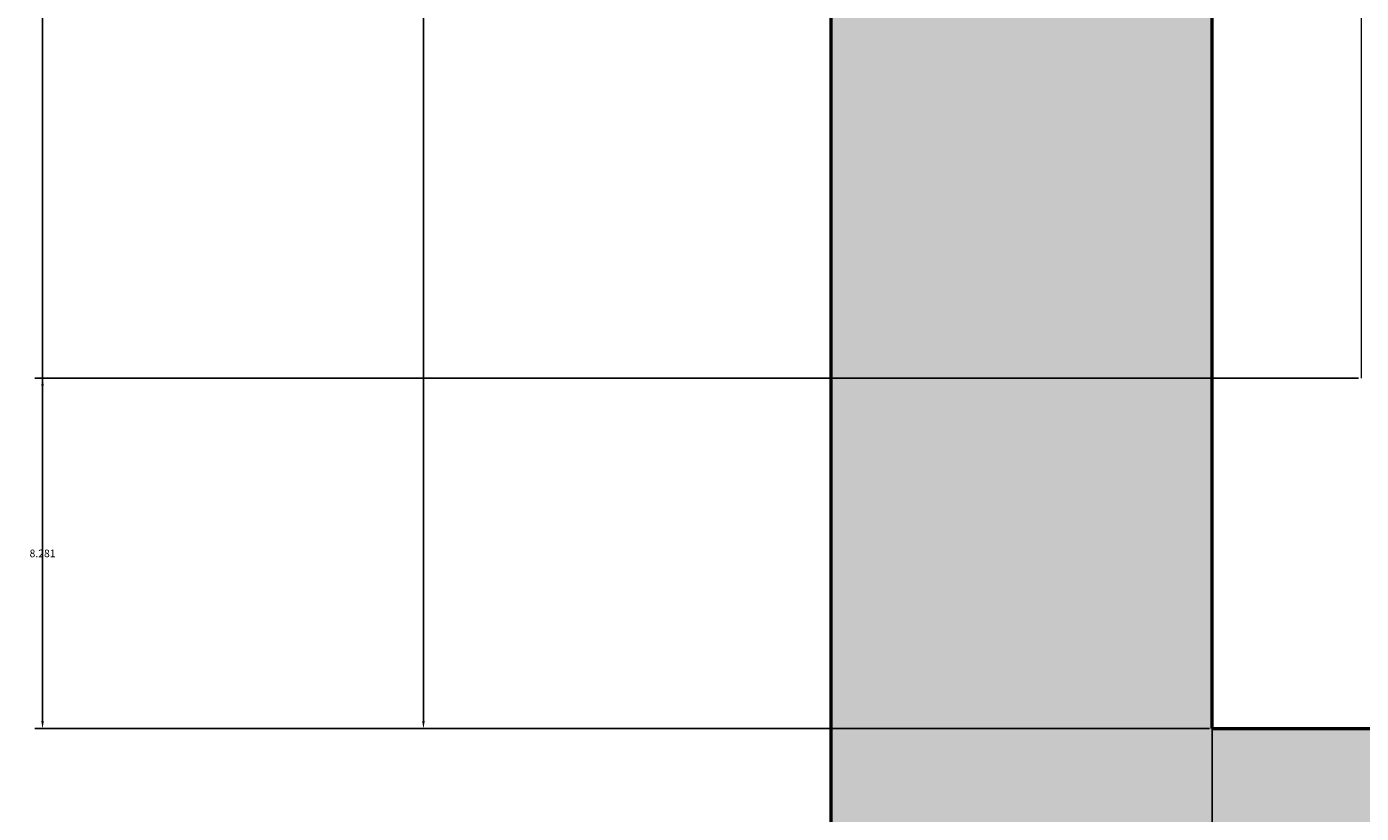
# Model space of a CAD drawing. Units: inches. Extents: x 2231 to 2461, y 2045 to 2455.
# Tile 36 of 95: x 2231 to 2262, y 2185 to 2203. Entities that reach past the tile are written whole.
import ezdxf

# ---------------------------------------------------------------- set-up
doc = ezdxf.new("R2010")
doc.units = ezdxf.units.IN
for name, color, linetype, lineweight in [('A-ANNO-DIMS', 2, 'Continuous', 18), ('A-FURN', 9, 'Continuous', 18), ('A-WALL', 7, 'Continuous', 50)]:
    doc.layers.add(name, color=color, linetype=linetype, lineweight=lineweight)
doc.layers.add('A-WALL-PATT', color=18, linetype='Continuous', lineweight=13, true_color=0x000000)
doc.styles.get("Standard").update_dxf_attribs({"font": 'arial.ttf'})
doc.dimstyles.get("Standard").update_dxf_attribs({"dimtxt": 0.18, "dimasz": 0.18, "dimexe": 0.18, "dimexo": 0.0625, "dimgap": 0.09, "dimtad": 0, "dimtih": 1, "dimtoh": 1, "dimdec": 4, "dimzin": 0, "dimdsep": 46, "dimtxsty": 'Standard', "dimcen": 0.09, "dimadec": 0, "dimazin": 0, "dimtfac": 1, "dimtdec": 4, "dimtofl": 0, "dimtmove": 0, "dimatfit": 3, "dimfxl": 1, "dimtolj": 1, "dimtzin": 0, "dimarcsym": 0})

# ---------------------------------------------------------------- blocks, each defined once
blk = doc.blocks.new('*D39')
at = {"layer": 'A-ANNO-DIMS', "color": 0, "lineweight": -2, "transparency": 16777216}
for p, q in [((2258.731, 2221.999), (2230.981, 2221.999)), ((2231.161, 2221.819), (2231.161, 2204.598)), ((2231.161, 2187.013), (2231.161, 2204.234)), ((2258.731, 2186.833), (2230.981, 2186.833))]:
    blk.add_line(p, q, dxfattribs=at)
at = {"layer": 'A-ANNO-DIMS', "color": 0, "transparency": 16777216}
for points in [[(2231.131, 2221.819), (2231.191, 2221.819), (2231.161, 2221.999)], [(2231.131, 2187.013), (2231.191, 2187.013), (2231.161, 2186.833)]]:
    blk.add_solid(points, dxfattribs=at)
at = {"layer": 'Defpoints', "color": 0, "transparency": 16777216}
for p in [(2231.161, 2221.999), (2258.794, 2221.999), (2258.794, 2186.833)]:
    blk.add_point(p, dxfattribs=at)
at = {"layer": 'A-ANNO-DIMS', "color": 0, "transparency": 16777216, "insert": (2231.161, 2204.416), "char_height": 0.18, "attachment_point": 5}
blk.add_mtext('\\A1;35.166', dxfattribs=at)
blk = doc.blocks.new('*D40')
at = {"layer": 'A-ANNO-DIMS', "color": 0, "lineweight": -2, "transparency": 16777216}
for p, q in [((2258.731, 2302.833), (2239.981, 2302.833)), ((2240.161, 2302.653), (2240.161, 2245.015)), ((2240.161, 2187.013), (2240.161, 2244.651)), ((2258.731, 2186.833), (2239.981, 2186.833))]:
    blk.add_line(p, q, dxfattribs=at)
at = {"layer": 'A-ANNO-DIMS', "color": 0, "transparency": 16777216}
for points in [[(2240.131, 2302.653), (2240.191, 2302.653), (2240.161, 2302.833)], [(2240.131, 2187.013), (2240.191, 2187.013), (2240.161, 2186.833)]]:
    blk.add_solid(points, dxfattribs=at)
at = {"layer": 'Defpoints', "color": 0, "transparency": 16777216}
for p in [(2240.161, 2302.833), (2258.794, 2302.833), (2258.794, 2186.833)]:
    blk.add_point(p, dxfattribs=at)
at = {"layer": 'A-ANNO-DIMS', "color": 0, "transparency": 16777216, "insert": (2240.161, 2244.833), "char_height": 0.18, "attachment_point": 5}
blk.add_mtext('\\A1;116', dxfattribs=at)
blk = doc.blocks.new('*D47')
at = {"layer": 'A-ANNO-DIMS', "color": 0, "lineweight": -2, "transparency": 16777216}
for p, q in [((2258.794, 2182.895), (2258.794, 2454.645)), ((2258.974, 2454.465), (2276.575, 2454.465)), ((2294.614, 2454.465), (2277.012, 2454.465)), ((2294.794, 2182.895), (2294.794, 2454.645))]:
    blk.add_line(p, q, dxfattribs=at)
at = {"layer": 'A-ANNO-DIMS', "color": 0, "transparency": 16777216}
for points in [[(2258.974, 2454.495), (2258.974, 2454.435), (2258.794, 2454.465)], [(2294.614, 2454.495), (2294.614, 2454.435), (2294.794, 2454.465)]]:
    blk.add_solid(points, dxfattribs=at)
at = {"layer": 'Defpoints', "color": 0, "transparency": 16777216}
for p in [(2294.794, 2454.465), (2258.794, 2182.833), (2294.794, 2182.833)]:
    blk.add_point(p, dxfattribs=at)
at = {"layer": 'A-ANNO-DIMS', "color": 0, "transparency": 16777216, "insert": (2276.794, 2454.465), "char_height": 0.18, "attachment_point": 5}
blk.add_mtext('\\A1;36', dxfattribs=at)
blk = doc.blocks.new('*D51')
at = {"layer": 'A-ANNO-DIMS', "color": 0, "lineweight": -2, "transparency": 16777216}
for p, q in [((2258.794, 2306.77), (2258.794, 2044.803)), ((2330.794, 2306.77), (2330.794, 2044.803)), ((2258.974, 2044.983), (2294.576, 2044.983)), ((2330.614, 2044.983), (2295.011, 2044.983))]:
    blk.add_line(p, q, dxfattribs=at)
at = {"layer": 'A-ANNO-DIMS', "color": 0, "transparency": 16777216}
for points in [[(2258.974, 2045.013), (2258.974, 2044.953), (2258.794, 2044.983)], [(2330.614, 2045.013), (2330.614, 2044.953), (2330.794, 2044.983)]]:
    blk.add_solid(points, dxfattribs=at)
at = {"layer": 'Defpoints', "color": 0, "transparency": 16777216}
for p in [(2258.794, 2306.833), (2330.794, 2306.833), (2330.794, 2044.983)]:
    blk.add_point(p, dxfattribs=at)
at = {"layer": 'A-ANNO-DIMS', "color": 0, "transparency": 16777216, "insert": (2294.794, 2044.983), "char_height": 0.18, "attachment_point": 5}
blk.add_mtext('\\A1;72', dxfattribs=at)
blk = doc.blocks.new('*D75')
at = {"layer": 'A-ANNO-DIMS', "color": 0, "lineweight": -2, "transparency": 16777216}
for p, q in [((2262.258, 2195.114), (2230.981, 2195.114)), ((2231.161, 2194.934), (2231.161, 2191.155)), ((2231.161, 2187.013), (2231.161, 2190.791)), ((2258.731, 2186.833), (2230.981, 2186.833))]:
    blk.add_line(p, q, dxfattribs=at)
at = {"layer": 'A-ANNO-DIMS', "color": 0, "transparency": 16777216}
for points in [[(2231.131, 2194.934), (2231.191, 2194.934), (2231.161, 2195.114)], [(2231.131, 2187.013), (2231.191, 2187.013), (2231.161, 2186.833)]]:
    blk.add_solid(points, dxfattribs=at)
at = {"layer": 'Defpoints', "color": 0, "transparency": 16777216}
for p in [(2231.161, 2195.114), (2262.321, 2195.114), (2258.794, 2186.833)]:
    blk.add_point(p, dxfattribs=at)
at = {"layer": 'A-ANNO-DIMS', "color": 0, "transparency": 16777216, "insert": (2231.161, 2190.973), "char_height": 0.18, "attachment_point": 5}
blk.add_mtext('\\A1;8.281', dxfattribs=at)

msp = doc.modelspace()

# ---------------------------------------------------------------- hatches: boundary and pattern name
at = {"layer": 'A-WALL-PATT'}
h = msp.add_hatch(color=256, dxfattribs=at)
h.dxf.hatch_style = 1
h.paths.add_polyline_path([(2441.7935, 2269.1535), (2432.7935, 2269.1535), (2432.7935, 2186.8328), (2396.7935, 2186.8328), (2396.7935, 2286.8328), (2394.7935, 2286.8328), (2394.7935, 2186.8328), (2334.7935, 2186.8328), (2334.7935, 2182.8328), (2432.7935, 2182.8328), (2432.7935, 2072.8328), (2416.6639, 2072.8328), (2416.6639, 2063.8328), (2441.7935, 2063.8328)])
h.paths.add_polyline_path([(2368.6639, 2072.8328), (2367.04, 2072.8328), (2330.7942, 2072.8328), (2330.7397, 2063.8328), (2368.6639, 2063.8328)])
h.paths.add_polyline_path([(2300.7392, 2068.3328), (2300.7392, 2072.8328), (2298.7935, 2072.8328), (2294.7935, 2072.8328), (2258.7935, 2072.8328), (2258.7935, 2120.8328), (2294.7935, 2120.8328), (2298.7935, 2120.8328), (2298.7935, 2128.8328), (2294.7935, 2128.8328), (2294.7935, 2124.8328), (2258.7935, 2124.8328), (2258.7935, 2182.8328), (2294.7935, 2182.8328), (2294.7935, 2174.8328), (2298.7935, 2174.8328), (2298.7935, 2182.8328), (2304.7935, 2182.8328), (2304.7935, 2186.8328), (2258.7935, 2186.8328), (2258.7935, 2221.999), (2249.7935, 2221.999), (2249.7935, 2063.8328), (2300.7392, 2063.8328)])
h.paths.add_polyline_path([(2391.9338, 2435.8328), (2333.82, 2435.8328), (2333.82, 2426.8328), (2368.7935, 2426.8328), (2368.7935, 2374.9508), (2368.7935, 2370.8328), (2372.3935, 2370.8328), (2372.7935, 2370.8328), (2372.7935, 2426.8328), (2391.9338, 2426.8328)])
h.paths.add_polyline_path([(2441.7935, 2435.8328), (2415.9338, 2435.8328), (2415.9338, 2426.8328), (2432.7935, 2426.8328), (2432.7935, 2334.8328), (2372.7935, 2334.8328), (2372.7935, 2346.8328), (2368.7935, 2346.8328), (2368.7935, 2306.8328), (2360.7935, 2306.8328), (2360.7935, 2302.8328), (2368.7935, 2302.8328), (2372.7935, 2302.8328), (2372.7935, 2330.8328), (2432.7935, 2330.8328), (2432.7935, 2317.1535), (2441.7935, 2317.1535)])
h.paths.add_polyline_path([(2285.82, 2435.8328), (2249.7935, 2435.8328), (2249.7935, 2269.999), (2258.7935, 2269.999), (2258.7935, 2302.8328), (2318.8168, 2302.8328), (2330.7935, 2302.8328), (2330.7935, 2306.8328), (2258.7935, 2306.8328), (2258.7935, 2426.8328), (2285.82, 2426.8328)])

# ---------------------------------------------------------------- linework, layer by layer
at = {"layer": 'A-FURN'}
msp.add_line((2262.3207, 2255.1137), (2262.3207, 2195.1137), dxfattribs=at)
at = {"layer": 'A-WALL'}
for q in [(2258.7935, 2302.8328), (2304.7935, 2186.8328)]:
    msp.add_line((2258.7935, 2186.8328), q, dxfattribs=at)
msp.add_lwpolyline([(2300.7392, 2063.8328), (2249.7935, 2063.8328), (2249.7935, 2435.8328), (2441.7935, 2435.8328), (2441.7935, 2063.8328), (2330.7397, 2063.8328)], dxfattribs=at)

# ---------------------------------------------------------------- dimensions: what is measured, and where the dimension line sits
at = {"layer": 'A-ANNO-DIMS'}
for base, p1, p2, picture, middle in [((2294.7935, 2454.4653), (2258.7935, 2182.8328), (2294.7935, 2182.8328), '*D47', (2276.7935, 2454.4653)), ((2330.7935, 2044.9825), (2258.7935, 2306.8328), (2330.7935, 2306.8328), '*D51', (2294.7935, 2044.9825))]:
    dim = msp.add_linear_dim(base=base, p1=p1, p2=p2, dimstyle='Standard', override={"dimdec": 0, "dimlfac": 1, "dimrnd": 0, "dimzin": 0, "dimdsep": 46, "dimlunit": 2}, dxfattribs=at)
    dim.commit()
    dim.dimension.update_dxf_attribs({"geometry": picture, "text_midpoint": middle})
for base, p2, override, picture, middle in [((2240.161, 2302.8328), (2258.7935, 2302.8328), {"dimdec": 0, "dimlfac": 1, "dimrnd": 0, "dimzin": 0, "dimdsep": 46, "dimlunit": 2}, '*D40', (2240.161, 2244.8328)), ((2231.161, 2221.999), (2258.7935, 2221.999), {"dimdec": 3, "dimlfac": 1, "dimrnd": 0, "dimzin": 0, "dimdsep": 46, "dimlunit": 2}, '*D39', (2231.161, 2204.4159)), ((2231.161, 2195.1137), (2262.3207, 2195.1137), {"dimdec": 3, "dimlfac": 1, "dimrnd": 0, "dimzin": 0, "dimdsep": 46, "dimlunit": 2}, '*D75', (2231.161, 2190.9733))]:
    dim = msp.add_linear_dim(base=base, p1=(2258.7935, 2186.8328), p2=p2, angle=90, dimstyle='Standard', override=override, dxfattribs=at)
    dim.commit()
    dim.dimension.update_dxf_attribs({"geometry": picture, "text_midpoint": middle})

doc.saveas('drawing.dxf')
